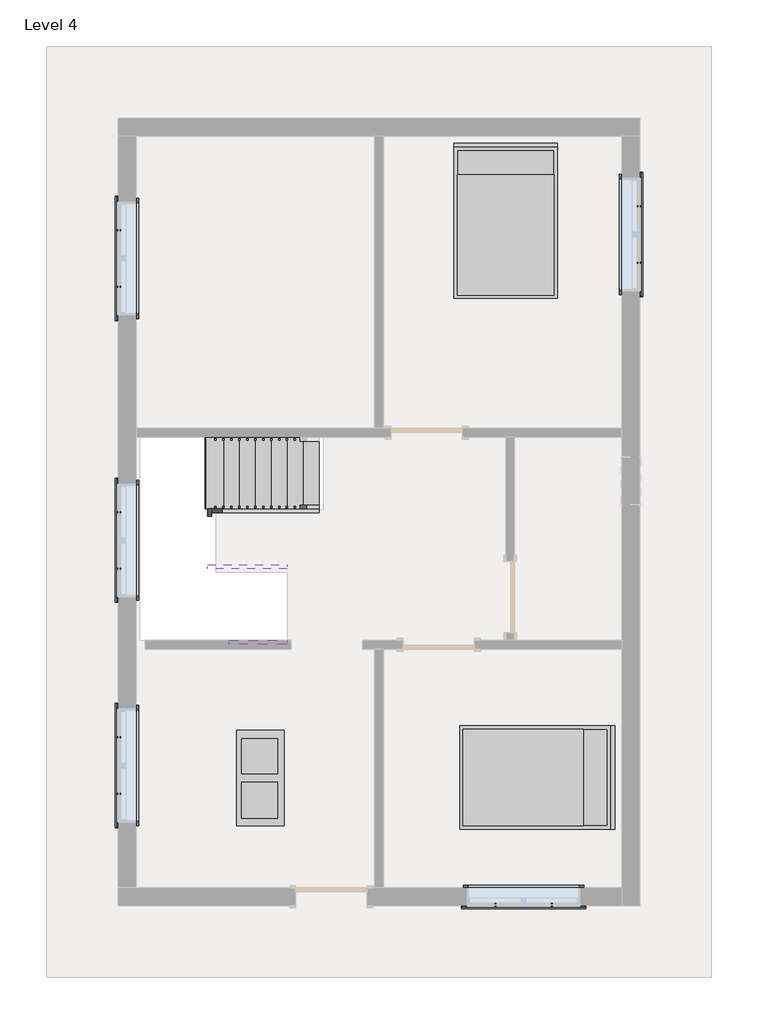
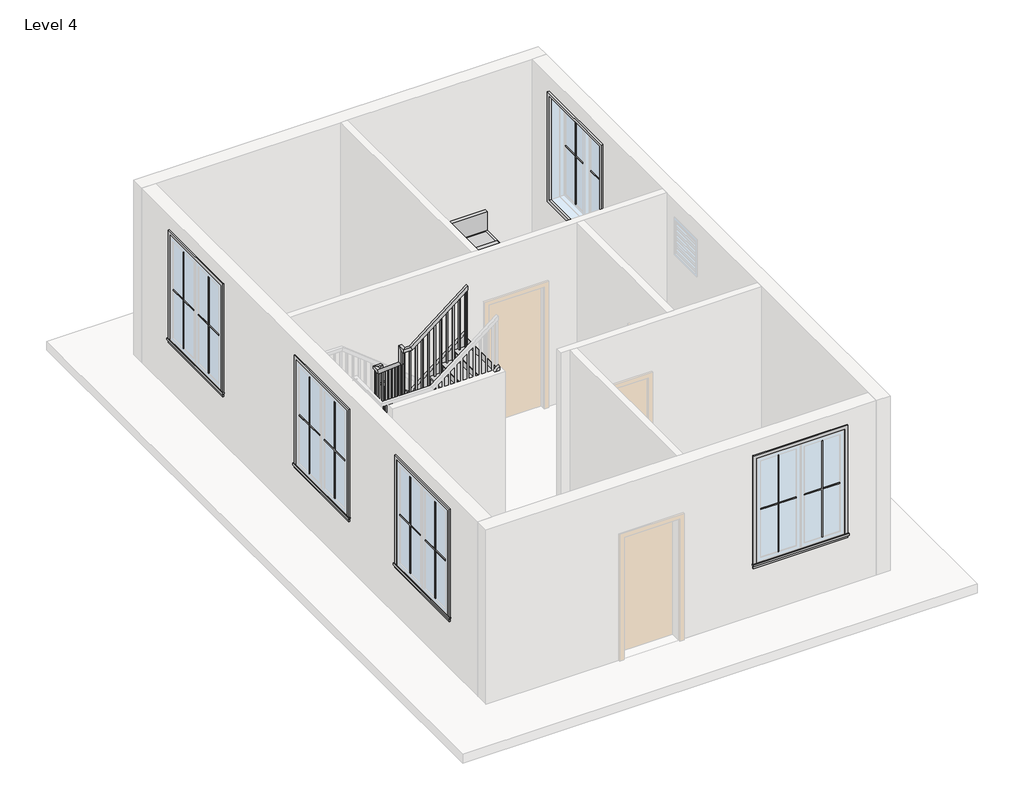
# One storey, part 2 of 2: 21 proxies, 5 members, 2 furniture elements, 1 railing, 1 stair flight.
"""IFC4 building model written with IfcOpenShell, lengths in millimetres."""

from ifc_helpers import new_model, si_unit, frame, origin, place, context, project, spatial, polyline, outline, extrude, faceted_brep, transform, mapped, element, save
from components import muntin_pattern_2x2_muntin_pattern_2x2_bff912c5, muntin_pattern_2x2_muntin_pattern_2x2_c2194282, trim_window_exterior_flat_with_sill_e04b3088, trim_window_interior_flat_picture_frame_2a7685fe, coffee_table_with_brass_mullions_11320_coffee_table_with_5962bef7, bed_17739_bed_17739_15c61121, stair_flight_50364206

model = new_model("IFC4")

# Units and contexts
model_context = context("Model", 3, world=origin())
ifc_project = project(units=[si_unit("LENGTHUNIT", "METRE", prefix="MILLI")], contexts=[model_context])

# Site, building, storey
site = spatial("IfcSite", under=ifc_project)
building = spatial("IfcBuilding", under=site)
storey = spatial("IfcBuildingStorey", under=building, Name="Level 4", Elevation=6400.8)

# Proxies
placement = place(None, origin())
muntin_pattern_2x2_muntin_pattern_2x2_shape = muntin_pattern_2x2_muntin_pattern_2x2_bff912c5(model_context)
element("IfcBuildingElementProxy", 1, Name="Muntin Pattern_2x2 : Muntin Pattern_2x2", ObjectType="Muntin Pattern_2x2 : Muntin Pattern_2x2", at=placement, inside=storey, context=model_context, shape_type="MappedRepresentation", body=[
    mapped(muntin_pattern_2x2_muntin_pattern_2x2_shape, transform((-626.5715247, -5050.1430046, 7385.05), x_axis=(-1.0, 0.0, 0.0), y_axis=(0.0, -1.0, 0.0), z_axis=(0.0, 0.0, 1.0))),
])
element("IfcBuildingElementProxy", 2, Name="Muntin Pattern_2x2 : Muntin Pattern_2x2", ObjectType="Muntin Pattern_2x2 : Muntin Pattern_2x2", at=placement, inside=storey, context=model_context, shape_type="MappedRepresentation", body=[
    mapped(muntin_pattern_2x2_muntin_pattern_2x2_shape, transform((-6159.0090247, -3629.3305046, 7385.05), x_axis=(0.0, 1.0, 0.0), y_axis=(-1.0, 0.0, 0.0), z_axis=(0.0, 0.0, 1.0))),
])
element("IfcBuildingElementProxy", 3, Name="Muntin Pattern_2x2 : Muntin Pattern_2x2", ObjectType="Muntin Pattern_2x2 : Muntin Pattern_2x2", at=placement, inside=storey, context=model_context, shape_type="MappedRepresentation", body=[
    mapped(muntin_pattern_2x2_muntin_pattern_2x2_shape, transform((489.4409753, 3873.1944954, 7385.05), x_axis=(0.0, -1.0, 0.0), y_axis=(1.0, 0.0, 0.0), z_axis=(0.0, 0.0, 1.0))),
])
element("IfcBuildingElementProxy", 4, Name="Muntin Pattern_2x2 : Muntin Pattern_2x2", ObjectType="Muntin Pattern_2x2 : Muntin Pattern_2x2", at=placement, inside=storey, context=model_context, shape_type="MappedRepresentation", body=[
    mapped(muntin_pattern_2x2_muntin_pattern_2x2_shape, transform((-6159.0090247, 2847.6694954, 7385.05), x_axis=(0.0, 1.0, 0.0), y_axis=(-1.0, 0.0, 0.0), z_axis=(0.0, 0.0, 1.0))),
])
element("IfcBuildingElementProxy", 5, Name="Muntin Pattern_2x2 : Muntin Pattern_2x2", ObjectType="Muntin Pattern_2x2 : Muntin Pattern_2x2", at=placement, inside=storey, context=model_context, shape_type="MappedRepresentation", body=[
    mapped(muntin_pattern_2x2_muntin_pattern_2x2_shape, transform((-6159.0090247, -752.7805046, 7385.05), x_axis=(0.0, 1.0, 0.0), y_axis=(-1.0, 0.0, 0.0), z_axis=(0.0, 0.0, 1.0))),
])
muntin_pattern_2x2_muntin_pattern_2x2_2_shape = muntin_pattern_2x2_muntin_pattern_2x2_c2194282(model_context)
element("IfcBuildingElementProxy", 6, Name="Muntin Pattern_2x2 : Muntin Pattern_2x2", ObjectType="Muntin Pattern_2x2 : Muntin Pattern_2x2", at=placement, inside=storey, context=model_context, shape_type="MappedRepresentation", body=[
    mapped(muntin_pattern_2x2_muntin_pattern_2x2_2_shape, transform((-1347.2965247, -5050.1430046, 7385.05), x_axis=(1.0, 0.0, 0.0), y_axis=(0.0, 1.0, 0.0), z_axis=(0.0, 0.0, 1.0))),
])
element("IfcBuildingElementProxy", 7, Name="Muntin Pattern_2x2 : Muntin Pattern_2x2", ObjectType="Muntin Pattern_2x2 : Muntin Pattern_2x2", at=placement, inside=storey, context=model_context, shape_type="MappedRepresentation", body=[
    mapped(muntin_pattern_2x2_muntin_pattern_2x2_2_shape, transform((-6159.0090247, -2908.6055046, 7385.05), x_axis=(0.0, -1.0, 0.0), y_axis=(1.0, 0.0, 0.0), z_axis=(0.0, 0.0, 1.0))),
])
element("IfcBuildingElementProxy", 8, Name="Muntin Pattern_2x2 : Muntin Pattern_2x2", ObjectType="Muntin Pattern_2x2 : Muntin Pattern_2x2", at=placement, inside=storey, context=model_context, shape_type="MappedRepresentation", body=[
    mapped(muntin_pattern_2x2_muntin_pattern_2x2_2_shape, transform((489.4409753, 3152.4694954, 7385.05), x_axis=(0.0, 1.0, 0.0), y_axis=(-1.0, 0.0, 0.0), z_axis=(0.0, 0.0, 1.0))),
])
element("IfcBuildingElementProxy", 9, Name="Muntin Pattern_2x2 : Muntin Pattern_2x2", ObjectType="Muntin Pattern_2x2 : Muntin Pattern_2x2", at=placement, inside=storey, context=model_context, shape_type="MappedRepresentation", body=[
    mapped(muntin_pattern_2x2_muntin_pattern_2x2_2_shape, transform((-6159.0090247, 3568.3944954, 7385.05), x_axis=(0.0, -1.0, 0.0), y_axis=(1.0, 0.0, 0.0), z_axis=(0.0, 0.0, 1.0))),
])
element("IfcBuildingElementProxy", 10, Name="Muntin Pattern_2x2 : Muntin Pattern_2x2", ObjectType="Muntin Pattern_2x2 : Muntin Pattern_2x2", at=placement, inside=storey, context=model_context, shape_type="MappedRepresentation", body=[
    mapped(muntin_pattern_2x2_muntin_pattern_2x2_2_shape, transform((-6159.0090247, -32.0555046, 7385.05), x_axis=(0.0, -1.0, 0.0), y_axis=(1.0, 0.0, 0.0), z_axis=(0.0, 0.0, 1.0))),
])
trim_window_exterior_flat_with_sill_shape = trim_window_exterior_flat_with_sill_e04b3088(model_context)
element("IfcBuildingElementProxy", 11, Name="Trim-Window-Exterior-Flat : with Sill", ObjectType="Trim-Window-Exterior-Flat : with Sill", at=placement, inside=storey, context=model_context, shape_type="MappedRepresentation", body=[
    mapped(trim_window_exterior_flat_with_sill_shape, transform((-986.9340247, -5059.6680046, 9144.0), x_axis=(1.0, 0.0, 0.0), y_axis=(0.0, 0.0, 1.0), z_axis=(0.0, -1.0, 0.0))),
])
element("IfcBuildingElementProxy", 12, Name="Trim-Window-Exterior-Flat : with Sill", ObjectType="Trim-Window-Exterior-Flat : with Sill", at=placement, inside=storey, context=model_context, shape_type="MappedRepresentation", body=[
    mapped(trim_window_exterior_flat_with_sill_shape, transform((-6168.5340247, -3268.9680046, 9144.0), x_axis=(0.0, -1.0, 0.0), y_axis=(0.0, 0.0, 1.0), z_axis=(-1.0, 0.0, 0.0))),
])
element("IfcBuildingElementProxy", 13, Name="Trim-Window-Exterior-Flat : with Sill", ObjectType="Trim-Window-Exterior-Flat : with Sill", at=placement, inside=storey, context=model_context, shape_type="MappedRepresentation", body=[
    mapped(trim_window_exterior_flat_with_sill_shape, transform((498.9659753, 3512.8319954, 9144.0), x_axis=(0.0, 1.0, 0.0), y_axis=(0.0, 0.0, 1.0), z_axis=(1.0, 0.0, 0.0))),
])
element("IfcBuildingElementProxy", 14, Name="Trim-Window-Exterior-Flat : with Sill", ObjectType="Trim-Window-Exterior-Flat : with Sill", at=placement, inside=storey, context=model_context, shape_type="MappedRepresentation", body=[
    mapped(trim_window_exterior_flat_with_sill_shape, transform((-6168.5340247, 3208.0319954, 9144.0), x_axis=(0.0, -1.0, 0.0), y_axis=(0.0, 0.0, 1.0), z_axis=(-1.0, 0.0, 0.0))),
])
element("IfcBuildingElementProxy", 15, Name="Trim-Window-Exterior-Flat : with Sill", ObjectType="Trim-Window-Exterior-Flat : with Sill", at=placement, inside=storey, context=model_context, shape_type="MappedRepresentation", body=[
    mapped(trim_window_exterior_flat_with_sill_shape, transform((-6168.5340247, -392.4180046, 9144.0), x_axis=(0.0, -1.0, 0.0), y_axis=(0.0, 0.0, 1.0), z_axis=(-1.0, 0.0, 0.0))),
])
trim_window_interior_flat_picture_frame_shape = trim_window_interior_flat_picture_frame_2a7685fe(model_context)
element("IfcBuildingElementProxy", 16, Name="Trim-Window-Interior-Flat : Picture Frame", ObjectType="Trim-Window-Interior-Flat : Picture Frame", at=placement, inside=storey, context=model_context, shape_type="MappedRepresentation", body=[
    mapped(trim_window_interior_flat_picture_frame_shape, transform((-986.9340247, -4831.0680046, 9144.0), x_axis=(-1.0, 0.0, 0.0), y_axis=(0.0, 0.0, 1.0), z_axis=(0.0, 1.0, 0.0))),
])
element("IfcBuildingElementProxy", 17, Name="Trim-Window-Interior-Flat : Picture Frame", ObjectType="Trim-Window-Interior-Flat : Picture Frame", at=placement, inside=storey, context=model_context, shape_type="MappedRepresentation", body=[
    mapped(trim_window_interior_flat_picture_frame_shape, transform((-5939.9340247, -3268.9680046, 9144.0), x_axis=(0.0, 1.0, 0.0), y_axis=(0.0, 0.0, 1.0), z_axis=(1.0, 0.0, 0.0))),
])
element("IfcBuildingElementProxy", 18, Name="Trim-Window-Interior-Flat : Picture Frame", ObjectType="Trim-Window-Interior-Flat : Picture Frame", at=placement, inside=storey, context=model_context, shape_type="MappedRepresentation", body=[
    mapped(trim_window_interior_flat_picture_frame_shape, transform((270.3659753, 3512.8319954, 9144.0), x_axis=(0.0, -1.0, 0.0), y_axis=(0.0, 0.0, 1.0), z_axis=(-1.0, 0.0, 0.0))),
])
element("IfcBuildingElementProxy", 19, Name="Trim-Window-Interior-Flat : Picture Frame", ObjectType="Trim-Window-Interior-Flat : Picture Frame", at=placement, inside=storey, context=model_context, shape_type="MappedRepresentation", body=[
    mapped(trim_window_interior_flat_picture_frame_shape, transform((-5939.9340247, 3208.0319954, 9144.0), x_axis=(0.0, 1.0, 0.0), y_axis=(0.0, 0.0, 1.0), z_axis=(1.0, 0.0, 0.0))),
])
element("IfcBuildingElementProxy", 20, Name="Trim-Window-Interior-Flat : Picture Frame", ObjectType="Trim-Window-Interior-Flat : Picture Frame", at=placement, inside=storey, context=model_context, shape_type="MappedRepresentation", body=[
    mapped(trim_window_interior_flat_picture_frame_shape, transform((-5939.9340247, -392.4180046, 9144.0), x_axis=(0.0, 1.0, 0.0), y_axis=(0.0, 0.0, 1.0), z_axis=(1.0, 0.0, 0.0))),
])
coffee_table_with_brass_mullions_11320_coffee_table_with_shape = coffee_table_with_brass_mullions_11320_coffee_table_with_5962bef7(model_context)
element("IfcBuildingElementProxy", 21, Name="coffee_table_with_brass_mullions_11320 : coffee_table_with_brass_mullions_11320", ObjectType="coffee_table_with_brass_mullions_11320 : coffee_table_with_brass_mullions_11320", at=placement, inside=storey, context=model_context, shape_type="MappedRepresentation", body=[
    mapped(coffee_table_with_brass_mullions_11320_coffee_table_with_shape, transform((-3920.6340247, -2792.7180046, 6400.8), x_axis=(0.0, 1.0, 0.0), y_axis=(-1.0, 0.0, 0.0), z_axis=(0.0, 0.0, 1.0))),
])

# Furniture
bed_17739_bed_17739_shape = bed_17739_bed_17739_15c61121(model_context)
element("IfcFurniture", 22, ObjectType="Bed_17739 : Bed_17739", at=placement, inside=storey, context=model_context, shape_type="MappedRepresentation", body=[
    mapped(bed_17739_bed_17739_shape, transform((-1215.5340247, 3665.2319954, 6400.8), x_axis=(1.0, 0.0, 0.0), y_axis=(0.0, 1.0, 0.0), z_axis=(0.0, 0.0, 1.0))),
])
element("IfcFurniture", 23, ObjectType="Bed_17739 : Bed_17739", at=placement, inside=storey, context=model_context, shape_type="MappedRepresentation", body=[
    mapped(bed_17739_bed_17739_shape, transform((-834.5340247, -3421.3680046, 6400.8), x_axis=(0.0, -1.0, 0.0), y_axis=(1.0, 0.0, 0.0), z_axis=(0.0, 0.0, 1.0))),
])

# Members
element("IfcMember", 24, ObjectType="Stringer - 2\" Width", at=placement, inside=storey, context=model_context, shape_type="SweptSolid", body=[
    extrude(outline(polyline([(6400.8, -3603.1340247), (6632.3686588, -3603.1340247), (7715.2107641, -4974.7340247), (7326.8725136, -4974.7340247), (6400.8, -3801.7088408), (6400.8, -3603.1340247)])), frame((0.0, -43.1680046, 0.0), z_axis=(0.0, 1.0, 0.0), x_axis=(0.0, 0.0, 1.0)), (0.0, 0.0, 1.0), 50.8),
])
element("IfcMember", 25, ObjectType="Stringer - 2\" Width", at=placement, inside=storey, context=model_context, shape_type="SweptSolid", body=[
    extrude(outline(polyline([(7.6319954, 7922.0930346), (7.6319954, 7523.6154064), (-703.5680046, 8122.5206696), (-703.5680046, 8520.9982978), (7.6319954, 7922.0930346)])), frame((-5025.5340247, 0.0, 0.0), z_axis=(1.0, 0.0, 0.0), x_axis=(0.0, 1.0, 0.0)), (0.0, 0.0, 1.0), 50.8),
])
element("IfcMember", 26, ObjectType="Stringer - 2\" Width", at=placement, inside=storey, context=model_context, shape_type="SweptSolid", body=[
    extrude(outline(polyline([(8717.842343, -5025.5340247), (8329.5040926, -5025.5340247), (9131.6093557, -4009.5340247), (9519.9476062, -4009.5340247), (8717.842343, -5025.5340247)])), frame((0.0, -754.3680046, 0.0), z_axis=(0.0, 1.0, 0.0), x_axis=(0.0, 0.0, 1.0)), (0.0, 0.0, 1.0), 50.8),
])
element("IfcMember", 27, ObjectType="Stringer - 2\" Width", at=placement, inside=storey, context=model_context, shape_type="SweptSolid", body=[
    extrude(outline(polyline([(6400.8, -3603.1340247), (6632.3686588, -3603.1340247), (7152.071982, -4261.4249007), (7152.071982, -4753.3200179), (6400.8, -3801.7088408), (6400.8, -3603.1340247)])), frame((0.0, 922.0319954, 0.0), z_axis=(0.0, 1.0, 0.0), x_axis=(0.0, 0.0, 1.0)), (0.0, 0.0, 1.0), 50.8),
])
element("IfcMember", 28, ObjectType="Stringer - 2\" Width", at=placement, inside=storey, context=model_context, shape_type="SweptSolid", body=[
    extrude(outline(polyline([(8935.3206696, -4258.1663605), (9131.6093557, -4009.5340247), (9519.9476062, -4009.5340247), (8935.3206696, -4750.0614777), (8935.3206696, -4258.1663605)])), frame((0.0, -1719.5680046, 0.0), z_axis=(0.0, 1.0, 0.0), x_axis=(0.0, 0.0, 1.0)), (0.0, 0.0, 1.0), 50.8),
])

# Railing
element("IfcRailing", 29, ObjectType="Handrail - Rectangular", at=placement, inside=storey, context=model_context, shape_type="SolidModel", body=[
    faceted_brep([(-3603.1340247, 7.6319954, 7475.6210526), (-3603.1340247, 7.6319954, 7410.8980109), (-3603.1340247, 58.4319954, 7410.8980109), (-3603.1340247, 58.4319954, 7475.6210526), (-4949.3340247, 7.6319954, 8538.4105263), (-5000.1340247, 7.6319954, 8513.7927477), (-5000.1340247, 58.4319954, 8513.7927477), (-4949.3340247, 58.4319954, 8538.4105263), (-4949.3340247, 7.6319954, 8823.1578947), (-5000.1340247, 7.6319954, 8772.3578947), (-5000.1340247, 58.4319954, 8772.3578947), (-4949.3340247, 58.4319954, 8823.1578947), (-5025.5340247, 7.6319954, 8823.1578947), (-5025.5340247, 7.6319954, 8772.3578947), (-5076.3340247, 58.4319954, 8772.3578947), (-5076.3340247, 58.4319954, 8823.1578947), (-5025.5340247, -68.5680046, 8823.1578947), (-5025.5340247, -87.1083685, 8772.3578947), (-5076.3340247, -87.1083685, 8772.3578947), (-5076.3340247, -68.5680046, 8823.1578947), (-5025.5340247, -678.1680046, 9336.5052632), (-5025.5340247, -728.9680046, 9312.8712725), (-5076.3340247, -728.9680046, 9312.8712725), (-5076.3340247, -678.1680046, 9336.5052632), (-5025.5340247, -678.1680046, 9621.2526316), (-5025.5340247, -728.9680046, 9570.4526316), (-5076.3340247, -728.9680046, 9570.4526316), (-5076.3340247, -678.1680046, 9621.2526316), (-5025.5340247, -754.3680046, 9621.2526316), (-5025.5340247, -754.3680046, 9570.4526316), (-5076.3340247, -805.1680046, 9570.4526316), (-5076.3340247, -805.1680046, 9621.2526316), (-4949.3340247, -754.3680046, 9621.2526316), (-4931.6981718, -754.3680046, 9570.4526316), (-4931.6981718, -805.1680046, 9570.4526316), (-4949.3340247, -805.1680046, 9621.2526316), (-4009.5340247, -754.3680046, 10363.2), (-4009.5340247, -805.1680046, 10363.2), (-4009.5340247, -805.1680046, 10298.4769583), (-4009.5340247, -754.3680046, 10298.4769583)], [[[0, 1, 2, 3]], [[1, 0, 4, 5]], [[2, 1, 5, 6]], [[3, 2, 6, 7]], [[0, 3, 7, 4]], [[5, 4, 8, 9]], [[6, 5, 9, 10]], [[7, 6, 10, 11]], [[4, 7, 11, 8]], [[9, 8, 12, 13]], [[10, 9, 13, 14]], [[11, 10, 14, 15]], [[8, 11, 15, 12]], [[13, 12, 16, 17]], [[14, 13, 17, 18]], [[15, 14, 18, 19]], [[12, 15, 19, 16]], [[17, 16, 20, 21]], [[18, 17, 21, 22]], [[19, 18, 22, 23]], [[16, 19, 23, 20]], [[21, 20, 24, 25]], [[22, 21, 25, 26]], [[23, 22, 26, 27]], [[20, 23, 27, 24]], [[25, 24, 28, 29]], [[26, 25, 29, 30]], [[27, 26, 30, 31]], [[24, 27, 31, 28]], [[29, 28, 32, 33]], [[30, 29, 33, 34]], [[31, 30, 34, 35]], [[28, 31, 35, 32]], [[36, 37, 38, 39]], [[33, 32, 36, 39]], [[34, 33, 39, 38]], [[35, 34, 38, 37]], [[32, 35, 37, 36]]]),
    extrude(outline(polyline([(10270.9045898, -4044.4590247), (9288.3789474, -4044.4590247), (9288.3789474, -4025.4090247), (10285.9440635, -4025.4090247), (10270.9045898, -4044.4590247)])), frame((0.0, -789.2930046, 0.0), z_axis=(0.0, 1.0, 0.0), x_axis=(0.0, 0.0, 1.0)), (0.0, 0.0, 1.0), 19.05),
    extrude(outline(polyline([(10190.6940635, -4146.0590247), (9288.3789474, -4146.0590247), (9288.3789474, -4127.0090247), (10205.7335372, -4127.0090247), (10190.6940635, -4146.0590247)])), frame((0.0, -789.2930046, 0.0), z_axis=(0.0, 1.0, 0.0), x_axis=(0.0, 0.0, 1.0)), (0.0, 0.0, 1.0), 19.05),
    extrude(outline(polyline([(10110.4835372, -4247.6590247), (9127.9578947, -4247.6590247), (9127.9578947, -4228.6090247), (10125.5230109, -4228.6090247), (10110.4835372, -4247.6590247)])), frame((0.0, -789.2930046, 0.0), z_axis=(0.0, 1.0, 0.0), x_axis=(0.0, 0.0, 1.0)), (0.0, 0.0, 1.0), 19.05),
    extrude(outline(polyline([(10030.2730109, -4349.2590247), (9127.9578947, -4349.2590247), (9127.9578947, -4330.2090247), (10045.3124846, -4330.2090247), (10030.2730109, -4349.2590247)])), frame((0.0, -789.2930046, 0.0), z_axis=(0.0, 1.0, 0.0), x_axis=(0.0, 0.0, 1.0)), (0.0, 0.0, 1.0), 19.05),
    extrude(outline(polyline([(9950.0624846, -4450.8590247), (8967.5368421, -4450.8590247), (8967.5368421, -4431.8090247), (9965.1019583, -4431.8090247), (9950.0624846, -4450.8590247)])), frame((0.0, -789.2930046, 0.0), z_axis=(0.0, 1.0, 0.0), x_axis=(0.0, 0.0, 1.0)), (0.0, 0.0, 1.0), 19.05),
    extrude(outline(polyline([(9869.8519583, -4552.4590247), (8967.5368421, -4552.4590247), (8967.5368421, -4533.4090247), (9884.8914319, -4533.4090247), (9869.8519583, -4552.4590247)])), frame((0.0, -789.2930046, 0.0), z_axis=(0.0, 1.0, 0.0), x_axis=(0.0, 0.0, 1.0)), (0.0, 0.0, 1.0), 19.05),
    extrude(outline(polyline([(9789.6414319, -4654.0590247), (8807.1157895, -4654.0590247), (8807.1157895, -4635.0090247), (9804.6809056, -4635.0090247), (9789.6414319, -4654.0590247)])), frame((0.0, -789.2930046, 0.0), z_axis=(0.0, 1.0, 0.0), x_axis=(0.0, 0.0, 1.0)), (0.0, 0.0, 1.0), 19.05),
    extrude(outline(polyline([(9709.4309056, -4755.6590247), (8807.1157895, -4755.6590247), (8807.1157895, -4736.6090247), (9724.4703793, -4736.6090247), (9709.4309056, -4755.6590247)])), frame((0.0, -789.2930046, 0.0), z_axis=(0.0, 1.0, 0.0), x_axis=(0.0, 0.0, 1.0)), (0.0, 0.0, 1.0), 19.05),
    extrude(outline(polyline([(9629.2203793, -4857.2590247), (8646.6947368, -4857.2590247), (8646.6947368, -4838.2090247), (9644.259853, -4838.2090247), (9629.2203793, -4857.2590247)])), frame((0.0, -789.2930046, 0.0), z_axis=(0.0, 1.0, 0.0), x_axis=(0.0, 0.0, 1.0)), (0.0, 0.0, 1.0), 19.05),
    extrude(outline(polyline([(9549.009853, -4958.8590247), (8646.6947368, -4958.8590247), (8646.6947368, -4939.8090247), (9564.0493267, -4939.8090247), (9549.009853, -4958.8590247)])), frame((0.0, -789.2930046, 0.0), z_axis=(0.0, 1.0, 0.0), x_axis=(0.0, 0.0, 1.0)), (0.0, 0.0, 1.0), 19.05),
    extrude(outline(polyline([(-668.6430046, 9262.0712725), (-668.6430046, 8325.8526316), (-687.6930046, 8325.8526316), (-687.6930046, 9278.1133778), (-668.6430046, 9262.0712725)])), frame((-5060.4590247, 0.0, 0.0), z_axis=(1.0, 0.0, 0.0), x_axis=(0.0, 1.0, 0.0)), (0.0, 0.0, 1.0), 19.05),
    extrude(outline(polyline([(-567.0430046, 9176.5133778), (-567.0430046, 8325.8526316), (-586.0930046, 8325.8526316), (-586.0930046, 9192.555483), (-567.0430046, 9176.5133778)])), frame((-5060.4590247, 0.0, 0.0), z_axis=(1.0, 0.0, 0.0), x_axis=(0.0, 1.0, 0.0)), (0.0, 0.0, 1.0), 19.05),
    extrude(outline(polyline([(-465.4430046, 9090.955483), (-465.4430046, 8165.4315789), (-484.4930046, 8165.4315789), (-484.4930046, 9106.9975883), (-465.4430046, 9090.955483)])), frame((-5060.4590247, 0.0, 0.0), z_axis=(1.0, 0.0, 0.0), x_axis=(0.0, 1.0, 0.0)), (0.0, 0.0, 1.0), 19.05),
    extrude(outline(polyline([(-363.8430046, 9005.3975883), (-363.8430046, 8165.4315789), (-382.8930046, 8165.4315789), (-382.8930046, 9021.4396935), (-363.8430046, 9005.3975883)])), frame((-5060.4590247, 0.0, 0.0), z_axis=(1.0, 0.0, 0.0), x_axis=(0.0, 1.0, 0.0)), (0.0, 0.0, 1.0), 19.05),
    extrude(outline(polyline([(-262.2430046, 8919.8396935), (-262.2430046, 8005.0105263), (-281.2930046, 8005.0105263), (-281.2930046, 8935.8817988), (-262.2430046, 8919.8396935)])), frame((-5060.4590247, 0.0, 0.0), z_axis=(1.0, 0.0, 0.0), x_axis=(0.0, 1.0, 0.0)), (0.0, 0.0, 1.0), 19.05),
    extrude(outline(polyline([(-160.6430046, 8834.2817988), (-160.6430046, 8005.0105263), (-179.6930046, 8005.0105263), (-179.6930046, 8850.3239041), (-160.6430046, 8834.2817988)])), frame((-5060.4590247, 0.0, 0.0), z_axis=(1.0, 0.0, 0.0), x_axis=(0.0, 1.0, 0.0)), (0.0, 0.0, 1.0), 19.05),
    extrude(outline(polyline([(-59.0430046, 8748.7239041), (-59.0430046, 7844.5894737), (-78.0930046, 7844.5894737), (-78.0930046, 8764.7660093), (-59.0430046, 8748.7239041)])), frame((-5060.4590247, 0.0, 0.0), z_axis=(1.0, 0.0, 0.0), x_axis=(0.0, 1.0, 0.0)), (0.0, 0.0, 1.0), 19.05),
    extrude(outline(polyline([(-5016.0090247, 23.5069954), (-5035.0590247, 23.5069954), (-5035.0590247, 42.5569954), (-5016.0090247, 42.5569954), (-5016.0090247, 23.5069954)])), frame((0.0, 0.0, 7684.1684211), z_axis=(0.0, 0.0, 1.0), x_axis=(1.0, 0.0, 0.0)), (0.0, 0.0, 1.0), 1088.1894737),
    extrude(outline(polyline([(8461.1545898, -4933.4590247), (7523.7473684, -4933.4590247), (7523.7473684, -4914.4090247), (8446.1151161, -4914.4090247), (8461.1545898, -4933.4590247)])), frame((0.0, 23.5069954, 0.0), z_axis=(0.0, 1.0, 0.0), x_axis=(0.0, 0.0, 1.0)), (0.0, 0.0, 1.0), 19.05),
    extrude(outline(polyline([(8380.9440635, -4831.8590247), (7523.7473684, -4831.8590247), (7523.7473684, -4812.8090247), (8365.9045898, -4812.8090247), (8380.9440635, -4831.8590247)])), frame((0.0, 23.5069954, 0.0), z_axis=(0.0, 1.0, 0.0), x_axis=(0.0, 0.0, 1.0)), (0.0, 0.0, 1.0), 19.05),
    extrude(outline(polyline([(8300.7335372, -4730.2590247), (7363.3263158, -4730.2590247), (7363.3263158, -4711.2090247), (8285.6940635, -4711.2090247), (8300.7335372, -4730.2590247)])), frame((0.0, 23.5069954, 0.0), z_axis=(0.0, 1.0, 0.0), x_axis=(0.0, 0.0, 1.0)), (0.0, 0.0, 1.0), 19.05),
    extrude(outline(polyline([(8220.5230109, -4628.6590247), (7363.3263158, -4628.6590247), (7363.3263158, -4609.6090247), (8205.4835372, -4609.6090247), (8220.5230109, -4628.6590247)])), frame((0.0, 23.5069954, 0.0), z_axis=(0.0, 1.0, 0.0), x_axis=(0.0, 0.0, 1.0)), (0.0, 0.0, 1.0), 19.05),
    extrude(outline(polyline([(8140.3124846, -4527.0590247), (7202.9052632, -4527.0590247), (7202.9052632, -4508.0090247), (8125.2730109, -4508.0090247), (8140.3124846, -4527.0590247)])), frame((0.0, 23.5069954, 0.0), z_axis=(0.0, 1.0, 0.0), x_axis=(0.0, 0.0, 1.0)), (0.0, 0.0, 1.0), 19.05),
    extrude(outline(polyline([(8060.1019583, -4425.4590247), (7202.9052632, -4425.4590247), (7202.9052632, -4406.4090247), (8045.0624846, -4406.4090247), (8060.1019583, -4425.4590247)])), frame((0.0, 23.5069954, 0.0), z_axis=(0.0, 1.0, 0.0), x_axis=(0.0, 0.0, 1.0)), (0.0, 0.0, 1.0), 19.05),
    extrude(outline(polyline([(7979.8914319, -4323.8590247), (7042.4842105, -4323.8590247), (7042.4842105, -4304.8090247), (7964.8519583, -4304.8090247), (7979.8914319, -4323.8590247)])), frame((0.0, 23.5069954, 0.0), z_axis=(0.0, 1.0, 0.0), x_axis=(0.0, 0.0, 1.0)), (0.0, 0.0, 1.0), 19.05),
    extrude(outline(polyline([(7899.6809056, -4222.2590247), (7042.4842105, -4222.2590247), (7042.4842105, -4203.2090247), (7884.6414319, -4203.2090247), (7899.6809056, -4222.2590247)])), frame((0.0, 23.5069954, 0.0), z_axis=(0.0, 1.0, 0.0), x_axis=(0.0, 0.0, 1.0)), (0.0, 0.0, 1.0), 19.05),
    extrude(outline(polyline([(7819.4703793, -4120.6590247), (6882.0631579, -4120.6590247), (6882.0631579, -4101.6090247), (7804.4309056, -4101.6090247), (7819.4703793, -4120.6590247)])), frame((0.0, 23.5069954, 0.0), z_axis=(0.0, 1.0, 0.0), x_axis=(0.0, 0.0, 1.0)), (0.0, 0.0, 1.0), 19.05),
    extrude(outline(polyline([(7739.259853, -4019.0590247), (6882.0631579, -4019.0590247), (6882.0631579, -4000.0090247), (7724.2203793, -4000.0090247), (7739.259853, -4019.0590247)])), frame((0.0, 23.5069954, 0.0), z_axis=(0.0, 1.0, 0.0), x_axis=(0.0, 0.0, 1.0)), (0.0, 0.0, 1.0), 19.05),
    extrude(outline(polyline([(7659.0493267, -3917.4590247), (6721.6421053, -3917.4590247), (6721.6421053, -3898.4090247), (7644.009853, -3898.4090247), (7659.0493267, -3917.4590247)])), frame((0.0, 23.5069954, 0.0), z_axis=(0.0, 1.0, 0.0), x_axis=(0.0, 0.0, 1.0)), (0.0, 0.0, 1.0), 19.05),
    extrude(outline(polyline([(7578.8388004, -3815.8590247), (6721.6421053, -3815.8590247), (6721.6421053, -3796.8090247), (7563.7993267, -3796.8090247), (7578.8388004, -3815.8590247)])), frame((0.0, 23.5069954, 0.0), z_axis=(0.0, 1.0, 0.0), x_axis=(0.0, 0.0, 1.0)), (0.0, 0.0, 1.0), 19.05),
    extrude(outline(polyline([(7498.628274, -3714.2590247), (6561.2210526, -3714.2590247), (6561.2210526, -3695.2090247), (7483.5888004, -3695.2090247), (7498.628274, -3714.2590247)])), frame((0.0, 23.5069954, 0.0), z_axis=(0.0, 1.0, 0.0), x_axis=(0.0, 0.0, 1.0)), (0.0, 0.0, 1.0), 19.05),
    extrude(outline(polyline([(-5041.4090247, -770.2430046), (-5041.4090247, -789.2930046), (-5060.4590247, -789.2930046), (-5060.4590247, -770.2430046), (-5041.4090247, -770.2430046)])), frame((0.0, 0.0, 8486.2736842), z_axis=(0.0, 0.0, 1.0), x_axis=(1.0, 0.0, 0.0)), (0.0, 0.0, 1.0), 1084.1789474),
    extrude(outline(polyline([(-5041.4090247, 23.5069954), (-5060.4590247, 23.5069954), (-5060.4590247, 42.5569954), (-5041.4090247, 42.5569954), (-5041.4090247, 23.5069954)])), frame((0.0, 0.0, 7684.1684211), z_axis=(0.0, 0.0, 1.0), x_axis=(1.0, 0.0, 0.0)), (0.0, 0.0, 1.0), 1088.1894737),
    extrude(outline(polyline([(10283.4374846, -4028.5840247), (9288.3789474, -4028.5840247), (9288.3789474, -4009.5340247), (10298.4769583, -4009.5340247), (10283.4374846, -4028.5840247)])), frame((0.0, -789.2930046, 0.0), z_axis=(0.0, 1.0, 0.0), x_axis=(0.0, 0.0, 1.0)), (0.0, 0.0, 1.0), 19.05),
    extrude(outline(polyline([(7425.9374846, -3622.1840247), (6561.2210526, -3622.1840247), (6561.2210526, -3603.1340247), (7410.8980109, -3603.1340247), (7425.9374846, -3622.1840247)])), frame((0.0, 23.5069954, 0.0), z_axis=(0.0, 1.0, 0.0), x_axis=(0.0, 0.0, 1.0)), (0.0, 0.0, 1.0), 19.05),
])

# Stair flight
stair_flight_shape = stair_flight_50364206(model_context)
element("IfcStairFlight", 30, ObjectType="2\" Tread 1\" Nosing 1/4\" Riser", at=placement, inside=storey, context=model_context, shape_type="MappedRepresentation", body=[
    mapped(stair_flight_shape, transform((0.0, 0.0, 0.0), x_axis=(1.0, 0.0, 0.0), y_axis=(0.0, 1.0, 0.0), z_axis=(0.0, 0.0, 1.0))),
])

save(model, "model.ifc")

# Revit data of these elements
# Type "Muntin Pattern_2x2 : Muntin Pattern_2x2"
#   Width [instance default] = 4' - 0"
#   Thickness = 0' - 0 1/2"
#   Height [instance default] = 4' - 0"
#   Distance = 0' - 0 3/4"
#   Interior Material [instance default] = none
#   Exterior Material [instance default] = none
#   Default Elevation = 0
# Type "Trim-Window-Exterior-Flat : with Sill"
#   Trim Width = 0' - 2 1/4"
#   Trim Thickness_Picture Frame = 0' - 1 1/4"
#   Trim Thickness_with Sill = 0' - 0 3/4"
#   Sill Thickness = 0' - 1 1/4"
#   Opening Width [instance default] = 2' - 0"
#   Opening Height [instance default] = 3' - 0"
#   Default Elevation = 4' - 0"
#   Sill = yes
#   Picture Frame = no
#   Trim Material [instance default] = none
# Type "Trim-Window-Interior-Flat : Picture Frame"
#   Trim Thickness_Picture Frame = 0' - 1 1/4"
#   Trim Width = 0' - 2 1/4"
#   Trim Thickness_with Sill = 0' - 0 3/4"
#   Sill Thickness = 0' - 1 1/4"
#   Opening Width [instance default] = 2' - 0"
#   Opening Height [instance default] = 3' - 0"
#   Default Elevation = 4' - 0"
#   Sill = no
#   Picture Frame = yes
#   Trim Material [instance default] = none
# Type "coffee_table_with_brass_mullions_11320 : coffee_table_with_brass_mullions_11320"
#   Default Elevation = 0
# Type "Bed_17739 : Bed_17739"
#   Default Elevation = 0
# Type "Handrail - Rectangular"
#   Assembly Code = "C2010400"
#   built-in parameter 1008612 = 0.0416667 (stored number, unit not read)
#   built-in parameter 1008611 = 0.0416667 (stored number, unit not read)
#   built-in parameter 1008609 = 0.333333 (stored number, unit not read)
#   built-in parameter 1008604 = 0.166667 (stored number, unit not read)
#   built-in parameter 1008603 = 0.166667 (stored number, unit not read)
#   Railing Height = 3' - 0"
#   built-in parameter 1008630 = 2
#   built-in parameter 1008610 = 2
#   built-in parameter 1008618 = Baluster - Square : 3/4"
# Elements 1, 2, 3, 4, 5, 6, 7, 8, 9, 10 (IfcBuildingElementProxy, "Muntin Pattern_2x2 : Muntin Pattern_2x2")
#   Width = 1' - 11 1/8"
#   Height = 5' - 6 1/2"
#   Interior Material = Wood - Stained
#   Exterior Material = Clad - White
#   Phase Created = New Construction
#   Materials on its faces: "Clad - White", "Wood - Stained"
# Elements 11, 12, 13, 14, 15 (IfcBuildingElementProxy, "Trim-Window-Exterior-Flat : with Sill")
#   Opening Width = 4' - 9"
#   Opening Height = 6' - 0"
#   Trim Material = Clad - White
#   Phase Created = New Construction
#   Materials on its faces: "Clad - White"
# Elements 16, 17, 18, 19, 20 (IfcBuildingElementProxy, "Trim-Window-Interior-Flat : Picture Frame")
#   Opening Width = 4' - 9"
#   Opening Height = 6' - 0"
#   Trim Material = Wood - Stained
#   Phase Created = New Construction
#   Materials on its faces: "Wood - Stained"
# Element 21 (IfcBuildingElementProxy, "coffee_table_with_brass_mullions_11320 : coffee_table_with_brass_mullions_11320")
#   Phase Created = New Construction
#   Materials on its faces: "Default Wall", "TABLE", "Glass", "Default"
# Elements 22, 23 (IfcFurniture, "Bed_17739 : Bed_17739")
#   Phase Created = New Construction
#   Materials on its faces: "legs", "sheets", "bed frame", "Blanket"
# Elements 24, 25, 26, 27, 28 (IfcMember, "Stringer - 2\" Width")
#   Phase Created = New Construction
# Element 29 (IfcRailing, "Handrail - Rectangular")
#   Phase Created = New Construction
#   Materials on its faces: "Oak Flooring"
# Element 30 (IfcStairFlight, "2\" Tread 1\" Nosing 1/4\" Riser")
#   Phase Created = New Construction
# Materials
#   "Clad - White": class "Wood", colour RGB 242 242 238, transparency 0, Cost = 0
#   "Wood - Stained": class "Wood", colour RGB 224 178 126, transparency 0, Cost = 0
#   "Default Wall": colour RGB 128 128 128, transparency 0, Cost = 0
#   "TABLE": class "Generic", colour RGB 120 120 120, transparency 0, Cost = 0
#   "Glass": class "Glass", colour RGB 0 128 192, transparency 0.75, Description = "Soda Lime Glass", Cost = 0
#   "Default": colour RGB 127 127 127, transparency 0, Cost = 0
#   "legs": colour RGB 90 73 37, transparency 0, Cost = 0
#   "sheets": colour RGB 200 195 176, transparency 0, Cost = 0
#   "bed frame": colour RGB 90 73 37, transparency 0, Cost = 0
#   "Blanket": class "System", colour RGB 59 0 1, transparency 0, Cost = 0
#   "Oak Flooring": class "Wood", colour RGB 216 169 114, transparency 0, Description = "Quercus Rubra", Cost = 0
